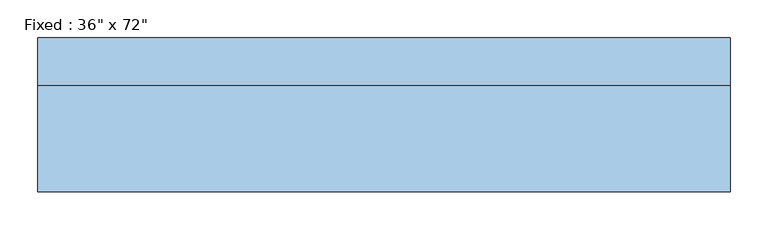
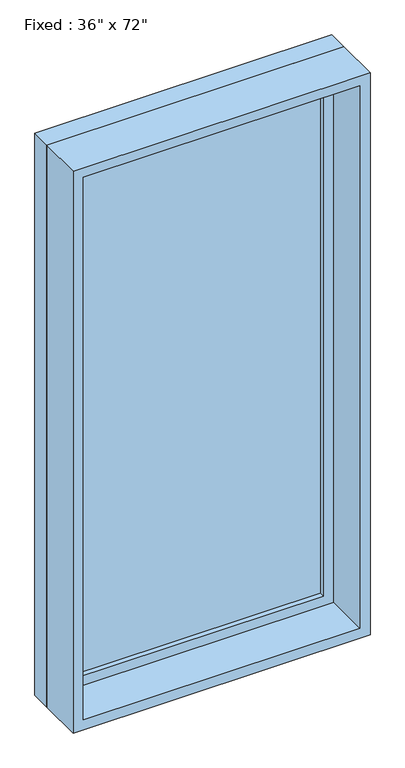
"""IFC4 building model written with IfcOpenShell, lengths in millimetres: window geometry."""

from ifc_helpers import new_model, si_unit, frame, origin, place, context, project, spatial, polyline, outline, extrude, source, transform, mapped, element, save


def window_9a779fa2(model_context):
    return source(origin(), model_context, "Body", "SweptSolid", [
        extrude(outline(polyline([(355.6, 53.975), (-431.8, 53.975), (-431.8, 66.675), (355.6, 66.675), (355.6, 53.975)])), frame((0.0, 0.0, 368.3), z_axis=(0.0, 0.0, 1.0), x_axis=(1.0, 0.0, 0.0)), (0.0, 0.0, 1.0), 1701.8),
        extrude(outline(polyline([(2114.55, -476.25), (323.85, -476.25), (323.85, 400.05), (2114.55, 400.05), (2114.55, -476.25)]), holes=[polyline([(2070.1, -431.8), (2070.1, 355.6), (368.3, 355.6), (368.3, -431.8), (2070.1, -431.8)])]), frame((0.0, 38.1, 0.0), z_axis=(0.0, 1.0, 0.0), x_axis=(0.0, 0.0, 1.0)), (0.0, 0.0, 1.0), 44.45),
        extrude(outline(polyline([(2133.6, -495.3), (304.8, -495.3), (304.8, 419.1), (2133.6, 419.1), (2133.6, -495.3)]), holes=[polyline([(2101.85, -463.55), (2101.85, 387.35), (336.55, 387.35), (336.55, -463.55), (2101.85, -463.55)])]), frame((0.0, -101.6, 0.0), z_axis=(0.0, 1.0, 0.0), x_axis=(0.0, 0.0, 1.0)), (0.0, 0.0, 1.0), 139.7),
        extrude(outline(polyline([(2133.6, 419.1), (2133.6, -495.3), (304.8, -495.3), (304.8, 419.1), (2133.6, 419.1)]), holes=[polyline([(2114.55, 400.05), (323.85, 400.05), (323.85, -476.25), (2114.55, -476.25), (2114.55, 400.05)])]), frame((0.0, 38.1, 0.0), z_axis=(0.0, 1.0, 0.0), x_axis=(0.0, 0.0, 1.0)), (0.0, 0.0, 1.0), 63.5),
    ])


if __name__ == "__main__":
    model = new_model("IFC4")
    model_context = context("Model", 3, world=origin())
    ifc_project = project(units=[si_unit("LENGTHUNIT", "METRE", prefix="MILLI")], contexts=[model_context])
    site = spatial("IfcSite", under=ifc_project)
    building = spatial("IfcBuilding", under=site)
    placement = place(None, origin())
    window_shape = window_9a779fa2(model_context)
    element("IfcWindow", 1, ObjectType="Fixed : 36\" x 72\"", at=placement, inside=building, context=model_context, shape_type="MappedRepresentation", body=[
        mapped(window_shape, transform((0.0, 0.0, 0.0), x_axis=(1.0, 0.0, 0.0), y_axis=(0.0, 1.0, 0.0), z_axis=(0.0, 0.0, 1.0))),
    ])
    save(model, "model.ifc")

# Revit data of these elements
# Type "Fixed : 36\" x 72\""
#   Type Mark = "9"
#   Construction Type Id = "GSP4R"
#   Assembly Code = "B2020100"
#   Analytic Construction = "1/8 in Pilkington single glazing"
#   Visual Light Transmittance = 0.9
#   Solar Heat Gain Coefficient = 0.78
#   Heat Transfer Coefficient (U) = 3.6886 W/(m²·K)
#   Height = 6' - 0"
#   Default Sill Height = 1' - 0"
#   Width = 3' - 0"
#   Window Inset = 0' - 0 3/4"
#   Glass Pane Material = Glass
#   Sash Material = Iron, Ductile
#   Wall Closure = (empty or 0)
# Element 1 (IfcWindow, "Fixed : 36\" x 72\"")
#   Materials on its faces: "Iron, Ductile", "Glass"
# Materials
#   "Glass": class "Glass", colour RGB 0 128 192, transparency 0.75, Description = "Soda Lime Glass", Cost = 0
#   "Iron, Ductile": class "Metal", colour RGB 0 0 0, transparency 0, Description = "Ductile cast iron", Cost = 0
